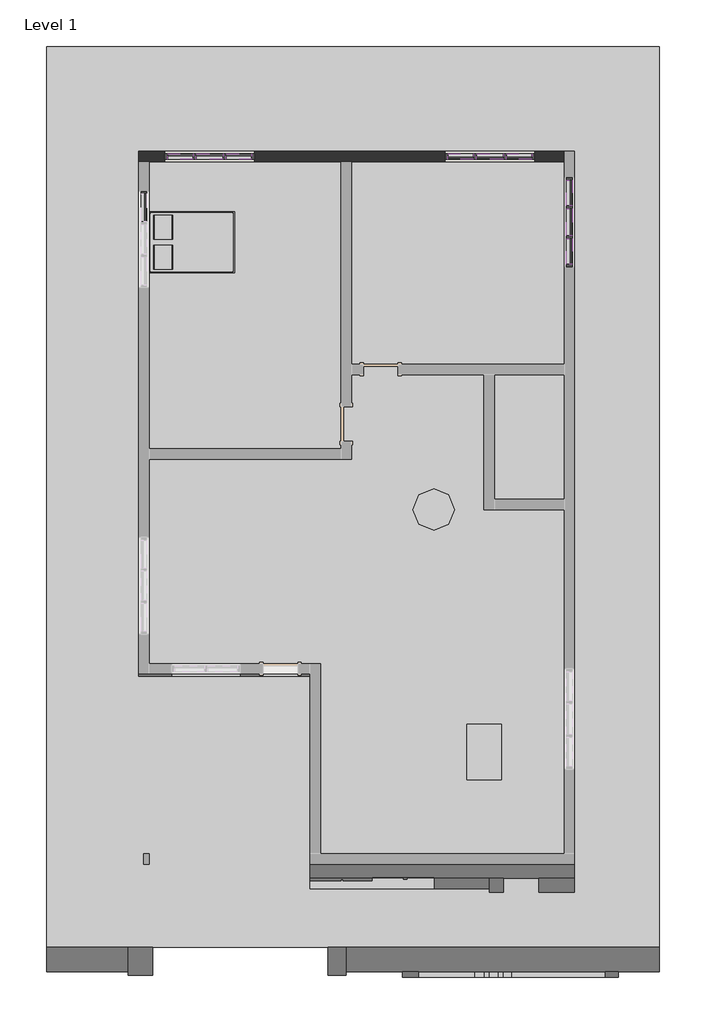
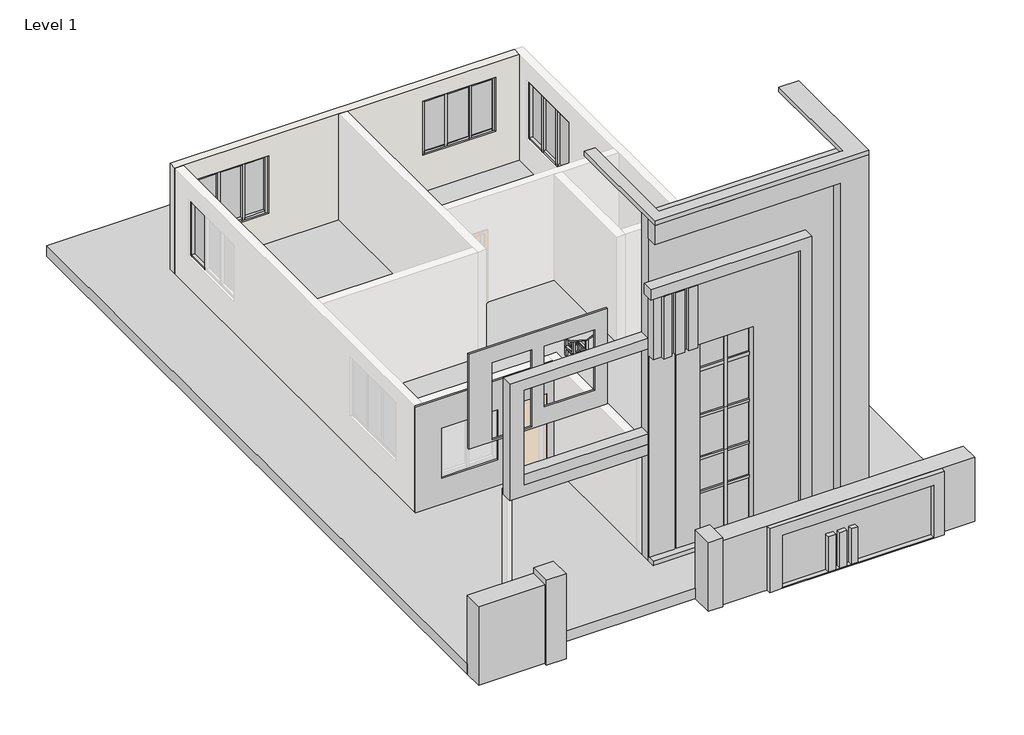
# One storey, part 2 of 2: 32 members, 10 plates, 3 furniture elements, 3 proxies, 1 wall.
"""IFC4 building model written with IfcOpenShell, lengths in millimetres."""

from ifc_helpers import new_model, si_unit, frame, origin, place, context, project, spatial, polyline, outline, extrude, faceted_brep, transform, mapped, element, save
from components import generic_models_1_generic_models_1_f513481b, generic_models_6_generic_models_6_42a028d1, furniture_b58f7881, furniture_acc2807d, furniture_52f35bf4, member_6f432376, member_a400357f, member_f14600c3, member_637ca32e, member_5ff6c43e, member_9389d775, member_1e31c4ff, member_d9b49a07, member_3f0e0172, member_8a463cd0, system_panel_glazed_0446ff67, system_panel_glazed_c50c6dba, system_panel_glazed_32442be8, system_panel_glazed_1c6e9dc7, system_panel_glazed_dfff3d37, system_panel_glazed_4691d008, system_panel_glazed_eebfb88d

model = new_model("IFC4")

# Units and contexts
model_context = context("Model", 3, world=origin())
ifc_project = project(units=[si_unit("LENGTHUNIT", "METRE", prefix="MILLI")], contexts=[model_context])

# Site, building, storey
site = spatial("IfcSite", under=ifc_project)
building = spatial("IfcBuilding", under=site)
storey = spatial("IfcBuildingStorey", under=building, Name="Level 1", Elevation=0.0)

# Proxies
placement = place(None, origin())
generic_models_1_generic_models_1_shape = generic_models_1_generic_models_1_f513481b(model_context)
element("IfcBuildingElementProxy", 1, Name="Generic Models 1 : Generic Models 1", ObjectType="Generic Models 1 : Generic Models 1", at=placement, inside=storey, context=model_context, shape_type="MappedRepresentation", body=[
    mapped(generic_models_1_generic_models_1_shape, transform((0.0, 0.0, 0.0), x_axis=(1.0, 0.0, 0.0), y_axis=(0.0, 1.0, 0.0), z_axis=(0.0, 0.0, 1.0))),
])
element("IfcBuildingElementProxy", 2, Name="Generic Models 2 : Generic Models 2", ObjectType="Generic Models 2 : Generic Models 2", at=placement, inside=storey, context=model_context, shape_type="SolidModel", body=[
    extrude(outline(polyline([(9822.6068762, -12103.529521), (9283.1169921, -12103.529521), (9283.1169921, -7061.629521), (0.0, -7061.629521), (0.0, -6274.229521), (9822.6068762, -6274.229521), (9822.6068762, -12103.529521)])), frame((0.0, -14950.4001929, 0.0), z_axis=(0.0, 1.0, 0.0), x_axis=(0.0, 0.0, 1.0)), (0.0, 0.0, 1.0), 304.8),
    extrude(outline(polyline([(8023.4485698, -12214.7903562), (7718.6485698, -12214.7903562), (7718.6485698, -8145.892021), (0.0, -8145.892021), (0.0, -7836.329521), (8023.4485698, -7836.329521), (8023.4485698, -12214.7903562)])), frame((0.0, -14950.4001929, 0.0), z_axis=(0.0, 1.0, 0.0), x_axis=(0.0, 0.0, 1.0)), (0.0, 0.0, 1.0), 304.8),
    faceted_brep([(-8153.829521, -14874.2001929, 7718.6485698), (-12103.529521, -14874.2001929, 7718.6485698), (-12103.529521, -14874.2001929, 5921.2879658), (-9360.329521, -14874.2001929, 5921.2879658), (-9360.329521, -14874.2001929, 130.0879658), (-12103.529521, -14874.2001929, 130.0879658), (-12103.529521, -14874.2001929, 0.0), (-8153.829521, -14874.2001929, 0.0), (-8153.829521, -14645.6001929, 7718.6485698), (-8153.829521, -14645.6001929, 0.0), (-12103.529521, -14645.6001929, 0.0), (-12103.529521, -14645.6001929, 7718.6485698), (-9360.329521, -14645.6001929, 130.0879658), (-9360.329521, -14645.6001929, 5921.2879658), (-10731.929521, -14645.6001929, 5921.2879658), (-10731.929521, -14645.6001929, 130.0879658), (-12103.529521, -14696.4001929, 130.0879658), (-12103.529521, -14696.4001929, 5921.2879658), (-11369.4072413, -14696.4001929, 5921.2879658), (-11369.4072413, -14696.4001929, 130.0879658), (-10731.929521, -14696.4001929, 130.0879658), (-10731.929521, -14696.4001929, 5921.2879658), (-11369.4072413, -14671.0001929, 130.0879658), (-11417.729521, -14671.0001929, 130.0879658), (-11417.729521, -14696.4001929, 130.0879658), (-11417.729521, -14696.4001929, 5921.2879658), (-11417.729521, -14671.0001929, 5921.2879658), (-11369.4072413, -14671.0001929, 5921.2879658)], [[[0, 1, 2, 3, 4, 5, 6, 7]], [[8, 9, 10, 11], [12, 13, 14, 15]], [[1, 0, 8, 11]], [[11, 10, 6, 5, 16, 17, 2, 1]], [[7, 6, 10, 9]], [[0, 7, 9, 8]], [[18, 19, 20, 21]], [[4, 3, 13, 12]], [[4, 12, 15, 20, 19, 22, 23, 24, 16, 5]], [[13, 3, 2, 17, 25, 26, 27, 18, 21, 14]], [[27, 26, 23, 22]], [[27, 22, 19, 18]], [[23, 26, 25, 24]], [[20, 15, 14, 21]], [[17, 16, 24, 25]]]),
    faceted_brep([(-6274.229521, -14645.6001929, 0.0), (-6274.229521, -14645.6001929, 9822.6068762), (-12103.529521, -14645.6001929, 9822.6068762), (-12103.529521, -14645.6001929, 0.0), (-9360.329521, -14645.6001929, 5921.2879658), (-9360.329521, -14645.6001929, 130.0879658), (-10731.929521, -14645.6001929, 130.0879658), (-10731.929521, -14645.6001929, 5921.2879658), (-6274.229521, -14340.8001929, 0.0), (-12103.529521, -14340.8001929, 0.0), (-12103.529521, -14340.8001929, 6400.8), (-12103.529521, -14340.8001929, 9822.6068762), (-6274.229521, -14340.8001929, 9822.6068762), (-6274.229521, -14340.8001929, 6400.8), (-9360.329521, -14620.2001929, 5921.2879658), (-10731.929521, -14620.2001929, 5921.2879658), (-10731.929521, -14620.2001929, 130.0879658), (-9360.329521, -14620.2001929, 130.0879658)], [[[0, 1, 2, 3], [4, 5, 6, 7]], [[8, 9, 10, 11, 12, 13]], [[1, 0, 8, 13, 12]], [[2, 1, 12, 11]], [[3, 2, 11, 10, 9]], [[0, 3, 9, 8]], [[14, 15, 16, 17]], [[14, 17, 5, 4]], [[17, 16, 6, 5]], [[16, 15, 7, 6]], [[15, 14, 4, 7]]]),
    extrude(outline(polyline([(-9969.4233324, -14671.0001929), (-10046.129521, -14671.0001929), (-10046.129521, -14620.2001929), (-9969.4233324, -14620.2001929), (-9969.4233324, -14671.0001929)])), frame((0.0, 0.0, 130.0879658), z_axis=(0.0, 0.0, 1.0), x_axis=(1.0, 0.0, 0.0)), (0.0, 0.0, 1.0), 5791.2),
    extrude(outline(polyline([(-9360.329521, -14671.0001929), (-10731.929521, -14671.0001929), (-10731.929521, -14620.2001929), (-9360.329521, -14620.2001929), (-9360.329521, -14671.0001929)])), frame((0.0, 0.0, 4975.7086338), z_axis=(0.0, 0.0, 1.0), x_axis=(1.0, 0.0, 0.0)), (0.0, 0.0, 1.0), 100.846843),
    extrude(outline(polyline([(-9360.329521, -14671.0001929), (-10731.929521, -14671.0001929), (-10731.929521, -14620.2001929), (-9360.329521, -14620.2001929), (-9360.329521, -14671.0001929)])), frame((0.0, 0.0, 3649.5165518), z_axis=(0.0, 0.0, 1.0), x_axis=(1.0, 0.0, 0.0)), (0.0, 0.0, 1.0), 71.0460044),
    extrude(outline(polyline([(-9360.329521, -14671.0001929), (-10731.929521, -14671.0001929), (-10731.929521, -14620.2001929), (-9360.329521, -14620.2001929), (-9360.329521, -14671.0001929)])), frame((0.0, 0.0, 2432.9915053), z_axis=(0.0, 0.0, 1.0), x_axis=(1.0, 0.0, 0.0)), (0.0, 0.0, 1.0), 63.6133902),
    extrude(outline(polyline([(-9360.329521, -14671.0001929), (-10731.929521, -14671.0001929), (-10731.929521, -14620.2001929), (-9360.329521, -14620.2001929), (-9360.329521, -14671.0001929)])), frame((0.0, 0.0, 1459.4738056), z_axis=(0.0, 0.0, 1.0), x_axis=(1.0, 0.0, 0.0)), (0.0, 0.0, 1.0), 65.6589833),
    extrude(outline(polyline([(-10945.1706491, -14975.8001929), (-11189.129521, -14975.8001929), (-11189.129521, -14874.2001929), (-10945.1706491, -14874.2001929), (-10945.1706491, -14975.8001929)])), frame((0.0, 0.0, 5921.2879658), z_axis=(0.0, 0.0, 1.0), x_axis=(1.0, 0.0, 0.0)), (0.0, 0.0, 1.0), 1797.360604),
    extrude(outline(polyline([(-11655.9903562, -14975.8001929), (-11874.929521, -14975.8001929), (-11874.929521, -14874.2001929), (-11655.9903562, -14874.2001929), (-11655.9903562, -14975.8001929)])), frame((0.0, 0.0, 5921.2879658), z_axis=(0.0, 0.0, 1.0), x_axis=(1.0, 0.0, 0.0)), (0.0, 0.0, 1.0), 1797.360604),
    extrude(outline(polyline([(-11297.3415593, -14975.8001929), (-11542.070497, -14975.8001929), (-11542.070497, -14874.2001929), (-11297.3415593, -14874.2001929), (-11297.3415593, -14975.8001929)])), frame((0.0, 0.0, 5921.2879658), z_axis=(0.0, 0.0, 1.0), x_axis=(1.0, 0.0, 0.0)), (0.0, 0.0, 1.0), 1797.360604),
    extrude(outline(polyline([(6096.0, -12103.529521), (6096.0, -15875.429521), (3352.8, -15875.429521), (3352.8, -12103.529521), (6096.0, -12103.529521)]), holes=[polyline([(3403.6, -15227.729521), (5613.4, -15227.729521), (5613.4, -14160.929521), (3403.6, -14160.929521), (3403.6, -15227.729521)]), polyline([(5594.0897089, -12446.429521), (3857.9365624, -12446.429521), (3857.9365624, -13818.029521), (5594.0897089, -13818.029521), (5594.0897089, -12446.429521)])]), frame((0.0, -12715.2001929, 0.0), z_axis=(0.0, 1.0, 0.0), x_axis=(0.0, 0.0, 1.0)), (0.0, 0.0, 1.0), 50.8),
    extrude(outline(polyline([(3048.0, -12103.529521), (3048.0, -15875.429521), (0.0, -15875.429521), (0.0, -12103.529521), (3048.0, -12103.529521)]), holes=[polyline([(2181.7525261, -13208.429521), (2181.7525261, -12294.029521), (50.8, -12294.029521), (50.8, -13208.429521), (2181.7525261, -13208.429521)]), polyline([(2181.7525261, -13627.529521), (750.5784943, -13627.529521), (750.5784943, -15151.529521), (2181.7525261, -15151.529521), (2181.7525261, -13627.529521)])]), frame((0.0, -10200.6001929, 0.0), z_axis=(0.0, 1.0, 0.0), x_axis=(0.0, 0.0, 1.0)), (0.0, 0.0, 1.0), 50.8),
    extrude(outline(polyline([(3352.8, -15487.5170157), (6096.0, -15487.5170157), (6096.0, -12103.529521), (6400.8, -12103.529521), (6400.8, -15875.429521), (3048.0, -15875.429521), (3048.0, -12103.529521), (3352.8, -12103.529521), (3352.8, -15487.5170157)])), frame((0.0, -14645.6001929, 0.0), z_axis=(0.0, 1.0, 0.0), x_axis=(0.0, 0.0, 1.0)), (0.0, 0.0, 1.0), 304.8),
    extrude(outline(polyline([(-12103.529521, -14340.8001929), (-12103.529521, -14645.6001929), (-15487.5170157, -14645.6001929), (-15487.5170157, -14340.8001929), (-12103.529521, -14340.8001929)])), frame((0.0, 0.0, 3352.8), z_axis=(0.0, 0.0, 1.0), x_axis=(1.0, 0.0, 0.0)), (0.0, 0.0, 1.0), 304.8),
])
generic_models_6_generic_models_6_shape = generic_models_6_generic_models_6_42a028d1(model_context)
element("IfcBuildingElementProxy", 3, Name="Generic Models 6 : Generic Models 6", ObjectType="Generic Models 6 : Generic Models 6", at=placement, inside=storey, context=model_context, shape_type="MappedRepresentation", body=[
    mapped(generic_models_6_generic_models_6_shape, transform((0.0, 0.0, 0.0), x_axis=(1.0, 0.0, 0.0), y_axis=(0.0, 1.0, 0.0), z_axis=(0.0, 0.0, 1.0))),
])

# Furniture
furniture_shape = furniture_b58f7881(model_context)
element("IfcFurniture", 4, ObjectType="Bed-Box : Double 53\" x 74\"", at=placement, inside=storey, context=model_context, shape_type="MappedRepresentation", body=[
    mapped(furniture_shape, transform((-14941.4590292, -989.3526519, 0.0), x_axis=(0.0, 1.0, 0.0), y_axis=(-1.0, 0.0, 0.0), z_axis=(0.0, 0.0, 1.0))),
])
furniture_2_shape = furniture_acc2807d(model_context)
element("IfcFurniture", 5, ObjectType="Table-Coffee Rectangular : 48\" x 30\"", at=placement, inside=storey, context=model_context, shape_type="MappedRepresentation", body=[
    mapped(furniture_2_shape, transform((-7898.5186892, -12477.6338232, 0.0), x_axis=(0.0, 1.0, 0.0), y_axis=(-1.0, 0.0, 0.0), z_axis=(0.0, 0.0, 1.0))),
])
furniture_3_shape = furniture_52f35bf4(model_context)
element("IfcFurniture", 6, ObjectType="Table-Dining Round w Chairs : 36\" Diameter", at=placement, inside=storey, context=model_context, shape_type="MappedRepresentation", body=[
    mapped(furniture_3_shape, transform((-9476.7114882, -6345.4215044, 0.0), x_axis=(1.0, 0.0, 0.0), y_axis=(0.0, 1.0, 0.0), z_axis=(0.0, 0.0, 1.0))),
])

# Members
member_shape = member_6f432376(model_context)
element("IfcMember", 7, ObjectType="Rectangular Mullion : 2.5\" x 5\" rectangular", at=placement, inside=storey, context=model_context, shape_type="MappedRepresentation", body=[
    mapped(member_shape, transform((-6388.529521, 156.2498071, 2498.2989313), x_axis=(0.0, 0.0, 1.0), y_axis=(-1.0, 0.0, 0.0), z_axis=(0.0, -1.0, 0.0))),
])
element("IfcMember", 8, ObjectType="Rectangular Mullion : 2.5\" x 5\" rectangular", at=placement, inside=storey, context=model_context, shape_type="MappedRepresentation", body=[
    mapped(member_shape, transform((-6388.529521, -1132.8001929, 2498.2989313), x_axis=(0.0, 0.0, 1.0), y_axis=(-1.0, 0.0, 0.0), z_axis=(0.0, -1.0, 0.0))),
])
element("IfcMember", 9, ObjectType="Rectangular Mullion : 2.5\" x 5\" rectangular", at=placement, inside=storey, context=model_context, shape_type="MappedRepresentation", body=[
    mapped(member_shape, transform((-7779.179521, 1242.0998071, 2608.4048272), x_axis=(0.0, 0.0, 1.0), y_axis=(0.0, 1.0, 0.0), z_axis=(-1.0, 0.0, 0.0))),
])
element("IfcMember", 10, ObjectType="Rectangular Mullion : 2.5\" x 5\" rectangular", at=placement, inside=storey, context=model_context, shape_type="MappedRepresentation", body=[
    mapped(member_shape, transform((-9068.229521, 1242.0998071, 2608.4048272), x_axis=(0.0, 0.0, 1.0), y_axis=(0.0, 1.0, 0.0), z_axis=(-1.0, 0.0, 0.0))),
])
element("IfcMember", 11, ObjectType="Rectangular Mullion : 2.5\" x 5\" rectangular", at=placement, inside=storey, context=model_context, shape_type="MappedRepresentation", body=[
    mapped(member_shape, transform((-14675.279521, 1242.0998071, 2518.5416429), x_axis=(0.0, 0.0, 1.0), y_axis=(0.0, -1.0, 0.0), z_axis=(1.0, 0.0, 0.0))),
])
element("IfcMember", 12, ObjectType="Rectangular Mullion : 2.5\" x 5\" rectangular", at=placement, inside=storey, context=model_context, shape_type="MappedRepresentation", body=[
    mapped(member_shape, transform((-13386.229521, 1242.0998071, 2518.5416429), x_axis=(0.0, 0.0, 1.0), y_axis=(0.0, -1.0, 0.0), z_axis=(1.0, 0.0, 0.0))),
])
member_2_shape = member_a400357f(model_context)
element("IfcMember", 13, ObjectType="Rectangular Mullion : 2.5\" x 5\" rectangular", at=placement, inside=storey, context=model_context, shape_type="MappedRepresentation", body=[
    mapped(member_2_shape, transform((-6388.529521, -504.1501929, 2498.2989313), x_axis=(0.0, 0.0, 1.0), y_axis=(-1.0, 0.0, 0.0), z_axis=(0.0, -1.0, 0.0))),
])
element("IfcMember", 14, ObjectType="Rectangular Mullion : 2.5\" x 5\" rectangular", at=placement, inside=storey, context=model_context, shape_type="MappedRepresentation", body=[
    mapped(member_2_shape, transform((-8439.579521, 1242.0998071, 2608.4048272), x_axis=(0.0, 0.0, 1.0), y_axis=(0.0, 1.0, 0.0), z_axis=(-1.0, 0.0, 0.0))),
])
element("IfcMember", 15, ObjectType="Rectangular Mullion : 2.5\" x 5\" rectangular", at=placement, inside=storey, context=model_context, shape_type="MappedRepresentation", body=[
    mapped(member_2_shape, transform((-14014.879521, 1242.0998071, 2518.5416429), x_axis=(0.0, 0.0, 1.0), y_axis=(0.0, -1.0, 0.0), z_axis=(1.0, 0.0, 0.0))),
])
member_3_shape = member_f14600c3(model_context)
element("IfcMember", 16, ObjectType="Rectangular Mullion : 2.5\" x 5\" rectangular", at=placement, inside=storey, context=model_context, shape_type="MappedRepresentation", body=[
    mapped(member_3_shape, transform((-6388.529521, 124.4998071, 812.0853055), x_axis=(0.0, -1.0, 0.0), y_axis=(-1.0, 0.0, 0.0), z_axis=(0.0, 0.0, -1.0))),
])
element("IfcMember", 17, ObjectType="Rectangular Mullion : 2.5\" x 5\" rectangular", at=placement, inside=storey, context=model_context, shape_type="MappedRepresentation", body=[
    mapped(member_3_shape, transform((-6388.529521, -535.9001929, 812.0853055), x_axis=(0.0, -1.0, 0.0), y_axis=(-1.0, 0.0, 0.0), z_axis=(0.0, 0.0, -1.0))),
])
element("IfcMember", 18, ObjectType="Rectangular Mullion : 2.5\" x 5\" rectangular", at=placement, inside=storey, context=model_context, shape_type="MappedRepresentation", body=[
    mapped(member_2_shape, transform((-6388.529521, 92.7498071, 812.0853055), x_axis=(0.0, 0.0, -1.0), y_axis=(-1.0, 0.0, 0.0), z_axis=(0.0, 1.0, 0.0))),
])
element("IfcMember", 19, ObjectType="Rectangular Mullion : 2.5\" x 5\" rectangular", at=placement, inside=storey, context=model_context, shape_type="MappedRepresentation", body=[
    mapped(member_2_shape, transform((-7842.679521, 1242.0998071, 1054.9476218), x_axis=(0.0, 0.0, -1.0), y_axis=(0.0, 1.0, 0.0), z_axis=(1.0, 0.0, 0.0))),
])
element("IfcMember", 20, ObjectType="Rectangular Mullion : 2.5\" x 5\" rectangular", at=placement, inside=storey, context=model_context, shape_type="MappedRepresentation", body=[
    mapped(member_2_shape, transform((-14611.779521, 1242.0998071, 854.6671361), x_axis=(0.0, 0.0, -1.0), y_axis=(0.0, -1.0, 0.0), z_axis=(-1.0, 0.0, 0.0))),
])
element("IfcMember", 21, ObjectType="Rectangular Mullion : 2.5\" x 5\" rectangular", at=placement, inside=storey, context=model_context, shape_type="MappedRepresentation", body=[
    mapped(member_shape, transform((-6388.529521, -567.6501929, 812.0853055), x_axis=(0.0, 0.0, -1.0), y_axis=(-1.0, 0.0, 0.0), z_axis=(0.0, 1.0, 0.0))),
])
element("IfcMember", 22, ObjectType="Rectangular Mullion : 2.5\" x 5\" rectangular", at=placement, inside=storey, context=model_context, shape_type="MappedRepresentation", body=[
    mapped(member_shape, transform((-6388.529521, 721.3998071, 812.0853055), x_axis=(0.0, 0.0, -1.0), y_axis=(-1.0, 0.0, 0.0), z_axis=(0.0, 1.0, 0.0))),
])
element("IfcMember", 23, ObjectType="Rectangular Mullion : 2.5\" x 5\" rectangular", at=placement, inside=storey, context=model_context, shape_type="MappedRepresentation", body=[
    mapped(member_shape, transform((-8503.079521, 1242.0998071, 1054.9476218), x_axis=(0.0, 0.0, -1.0), y_axis=(0.0, 1.0, 0.0), z_axis=(1.0, 0.0, 0.0))),
])
element("IfcMember", 24, ObjectType="Rectangular Mullion : 2.5\" x 5\" rectangular", at=placement, inside=storey, context=model_context, shape_type="MappedRepresentation", body=[
    mapped(member_shape, transform((-7214.029521, 1242.0998071, 1054.9476218), x_axis=(0.0, 0.0, -1.0), y_axis=(0.0, 1.0, 0.0), z_axis=(1.0, 0.0, 0.0))),
])
element("IfcMember", 25, ObjectType="Rectangular Mullion : 2.5\" x 5\" rectangular", at=placement, inside=storey, context=model_context, shape_type="MappedRepresentation", body=[
    mapped(member_shape, transform((-13951.379521, 1242.0998071, 854.6671361), x_axis=(0.0, 0.0, -1.0), y_axis=(0.0, -1.0, 0.0), z_axis=(-1.0, 0.0, 0.0))),
])
element("IfcMember", 26, ObjectType="Rectangular Mullion : 2.5\" x 5\" rectangular", at=placement, inside=storey, context=model_context, shape_type="MappedRepresentation", body=[
    mapped(member_shape, transform((-15240.429521, 1242.0998071, 854.6671361), x_axis=(0.0, 0.0, -1.0), y_axis=(0.0, -1.0, 0.0), z_axis=(-1.0, 0.0, 0.0))),
])
member_4_shape = member_637ca32e(model_context)
element("IfcMember", 27, ObjectType="Rectangular Mullion : 2.5\" x 5\" rectangular", at=placement, inside=storey, context=model_context, shape_type="MappedRepresentation", body=[
    mapped(member_4_shape, transform((-6388.529521, 784.8998071, 2498.2989313), x_axis=(0.0, 1.0, 0.0), y_axis=(-1.0, 0.0, 0.0), z_axis=(0.0, 0.0, 1.0))),
])
element("IfcMember", 28, ObjectType="Rectangular Mullion : 2.5\" x 5\" rectangular", at=placement, inside=storey, context=model_context, shape_type="MappedRepresentation", body=[
    mapped(member_4_shape, transform((-6388.529521, -1196.3001929, 812.0853055), x_axis=(0.0, -1.0, 0.0), y_axis=(-1.0, 0.0, 0.0), z_axis=(0.0, 0.0, -1.0))),
])
member_5_shape = member_5ff6c43e(model_context)
element("IfcMember", 29, ObjectType="Rectangular Mullion : 2.5\" x 5\" rectangular", at=placement, inside=storey, context=model_context, shape_type="MappedRepresentation", body=[
    mapped(member_5_shape, transform((-8471.329521, 1242.0998071, 1054.9476218), x_axis=(-1.0, 0.0, 0.0), y_axis=(0.0, 1.0, 0.0), z_axis=(0.0, 0.0, -1.0))),
])
element("IfcMember", 30, ObjectType="Rectangular Mullion : 2.5\" x 5\" rectangular", at=placement, inside=storey, context=model_context, shape_type="MappedRepresentation", body=[
    mapped(member_5_shape, transform((-7810.929521, 1242.0998071, 1054.9476218), x_axis=(-1.0, 0.0, 0.0), y_axis=(0.0, 1.0, 0.0), z_axis=(0.0, 0.0, -1.0))),
])
member_6_shape = member_9389d775(model_context)
element("IfcMember", 31, ObjectType="Rectangular Mullion : 2.5\" x 5\" rectangular", at=placement, inside=storey, context=model_context, shape_type="MappedRepresentation", body=[
    mapped(member_6_shape, transform((-9131.729521, 1242.0998071, 1054.9476218), x_axis=(-1.0, 0.0, 0.0), y_axis=(0.0, 1.0, 0.0), z_axis=(0.0, 0.0, -1.0))),
])
element("IfcMember", 32, ObjectType="Rectangular Mullion : 2.5\" x 5\" rectangular", at=placement, inside=storey, context=model_context, shape_type="MappedRepresentation", body=[
    mapped(member_6_shape, transform((-7150.529521, 1242.0998071, 2608.4048272), x_axis=(1.0, 0.0, 0.0), y_axis=(0.0, 1.0, 0.0), z_axis=(0.0, 0.0, 1.0))),
])
member_7_shape = member_1e31c4ff(model_context)
element("IfcMember", 33, ObjectType="Rectangular Mullion : 2.5\" x 5\" rectangular", at=placement, inside=storey, context=model_context, shape_type="MappedRepresentation", body=[
    mapped(member_7_shape, transform((-14643.529521, 1242.0998071, 854.6671361), x_axis=(1.0, 0.0, 0.0), y_axis=(0.0, -1.0, 0.0), z_axis=(0.0, 0.0, -1.0))),
])
element("IfcMember", 34, ObjectType="Rectangular Mullion : 2.5\" x 5\" rectangular", at=placement, inside=storey, context=model_context, shape_type="MappedRepresentation", body=[
    mapped(member_7_shape, transform((-13983.129521, 1242.0998071, 854.6671361), x_axis=(1.0, 0.0, 0.0), y_axis=(0.0, -1.0, 0.0), z_axis=(0.0, 0.0, -1.0))),
])
member_8_shape = member_d9b49a07(model_context)
element("IfcMember", 35, ObjectType="Rectangular Mullion : 2.5\" x 5\" rectangular", at=placement, inside=storey, context=model_context, shape_type="MappedRepresentation", body=[
    mapped(member_8_shape, transform((-15303.929521, 1242.0998071, 2518.5416429), x_axis=(-1.0, 0.0, 0.0), y_axis=(0.0, -1.0, 0.0), z_axis=(0.0, 0.0, 1.0))),
])
element("IfcMember", 36, ObjectType="Rectangular Mullion : 2.5\" x 5\" rectangular", at=placement, inside=storey, context=model_context, shape_type="MappedRepresentation", body=[
    mapped(member_8_shape, transform((-13322.729521, 1242.0998071, 854.6671361), x_axis=(1.0, 0.0, 0.0), y_axis=(0.0, -1.0, 0.0), z_axis=(0.0, 0.0, -1.0))),
])
member_9_shape = member_3f0e0172(model_context)
element("IfcMember", 37, ObjectType="Rectangular Mullion : 2.5\" x 5\" rectangular", at=placement, inside=storey, context=model_context, shape_type="MappedRepresentation", body=[
    mapped(member_9_shape, transform((-15761.129521, 416.5998071, 913.1300213), x_axis=(0.0, 0.0, -1.0), y_axis=(-1.0, 0.0, 0.0), z_axis=(0.0, 1.0, 0.0))),
])
member_10_shape = member_8a463cd0(model_context)
element("IfcMember", 38, ObjectType="Rectangular Mullion : 2.5\" x 5\" rectangular", at=placement, inside=storey, context=model_context, shape_type="MappedRepresentation", body=[
    mapped(member_10_shape, transform((-15761.129521, 480.0998071, 2533.943824), x_axis=(0.0, 1.0, 0.0), y_axis=(-1.0, 0.0, 0.0), z_axis=(0.0, 0.0, 1.0))),
])

# Plates
system_panel_glazed_shape = system_panel_glazed_0446ff67(model_context)
element("IfcPlate", 39, ObjectType="System Panel : Glazed", at=placement, inside=storey, context=model_context, shape_type="MappedRepresentation", body=[
    mapped(system_panel_glazed_shape, transform((-6388.529521, 438.8248071, 875.5853055), x_axis=(0.0, -1.0, 0.0), y_axis=(1.0, 0.0, 0.0), z_axis=(0.0, 0.0, 1.0))),
])
element("IfcPlate", 40, ObjectType="System Panel : Glazed", at=placement, inside=storey, context=model_context, shape_type="MappedRepresentation", body=[
    mapped(system_panel_glazed_shape, transform((-6388.529521, -850.2251929, 875.5853055), x_axis=(0.0, -1.0, 0.0), y_axis=(1.0, 0.0, 0.0), z_axis=(0.0, 0.0, 1.0))),
])
system_panel_glazed_2_shape = system_panel_glazed_c50c6dba(model_context)
element("IfcPlate", 41, ObjectType="System Panel : Glazed", at=placement, inside=storey, context=model_context, shape_type="MappedRepresentation", body=[
    mapped(system_panel_glazed_2_shape, transform((-6388.529521, -205.7001929, 875.5853055), x_axis=(0.0, -1.0, 0.0), y_axis=(1.0, 0.0, 0.0), z_axis=(0.0, 0.0, 1.0))),
])
system_panel_glazed_3_shape = system_panel_glazed_32442be8(model_context)
element("IfcPlate", 42, ObjectType="System Panel : Glazed", at=placement, inside=storey, context=model_context, shape_type="MappedRepresentation", body=[
    mapped(system_panel_glazed_3_shape, transform((-7496.604521, 1242.0998071, 1118.4476218), x_axis=(-1.0, 0.0, 0.0), y_axis=(0.0, -1.0, 0.0), z_axis=(0.0, 0.0, 1.0))),
])
element("IfcPlate", 43, ObjectType="System Panel : Glazed", at=placement, inside=storey, context=model_context, shape_type="MappedRepresentation", body=[
    mapped(system_panel_glazed_3_shape, transform((-8785.654521, 1242.0998071, 1118.4476218), x_axis=(-1.0, 0.0, 0.0), y_axis=(0.0, -1.0, 0.0), z_axis=(0.0, 0.0, 1.0))),
])
system_panel_glazed_4_shape = system_panel_glazed_1c6e9dc7(model_context)
element("IfcPlate", 44, ObjectType="System Panel : Glazed", at=placement, inside=storey, context=model_context, shape_type="MappedRepresentation", body=[
    mapped(system_panel_glazed_4_shape, transform((-8141.129521, 1242.0998071, 1118.4476218), x_axis=(-1.0, 0.0, 0.0), y_axis=(0.0, -1.0, 0.0), z_axis=(0.0, 0.0, 1.0))),
])
system_panel_glazed_5_shape = system_panel_glazed_dfff3d37(model_context)
element("IfcPlate", 45, ObjectType="System Panel : Glazed", at=placement, inside=storey, context=model_context, shape_type="MappedRepresentation", body=[
    mapped(system_panel_glazed_5_shape, transform((-14957.854521, 1242.0998071, 918.1671361), x_axis=(1.0, 0.0, 0.0), y_axis=(0.0, 1.0, 0.0), z_axis=(0.0, 0.0, 1.0))),
])
element("IfcPlate", 46, ObjectType="System Panel : Glazed", at=placement, inside=storey, context=model_context, shape_type="MappedRepresentation", body=[
    mapped(system_panel_glazed_5_shape, transform((-13668.804521, 1242.0998071, 918.1671361), x_axis=(1.0, 0.0, 0.0), y_axis=(0.0, 1.0, 0.0), z_axis=(0.0, 0.0, 1.0))),
])
system_panel_glazed_6_shape = system_panel_glazed_4691d008(model_context)
element("IfcPlate", 47, ObjectType="System Panel : Glazed", at=placement, inside=storey, context=model_context, shape_type="MappedRepresentation", body=[
    mapped(system_panel_glazed_6_shape, transform((-14313.329521, 1242.0998071, 918.1671361), x_axis=(1.0, 0.0, 0.0), y_axis=(0.0, 1.0, 0.0), z_axis=(0.0, 0.0, 1.0))),
])
system_panel_glazed_7_shape = system_panel_glazed_eebfb88d(model_context)
element("IfcPlate", 48, ObjectType="System Panel : Glazed", at=placement, inside=storey, context=model_context, shape_type="MappedRepresentation", body=[
    mapped(system_panel_glazed_7_shape, transform((-15761.129521, 108.6248071, 976.6300213), x_axis=(0.0, -1.0, 0.0), y_axis=(1.0, 0.0, 0.0), z_axis=(0.0, 0.0, 1.0))),
])

# Wall
element("IfcWall", 49, ObjectType="9\"", at=placement, inside=storey, context=model_context, shape_type="Brep", body=[
    faceted_brep([(-6502.829521, 1356.3998071, 0.0), (-15875.429521, 1356.3998071, 0.0), (-15875.429521, 1356.3998071, 3048.0), (-6502.829521, 1356.3998071, 3048.0), (-7150.529521, 1356.3998071, 1054.9476218), (-7150.529521, 1356.3998071, 2608.4048272), (-9131.729521, 1356.3998071, 2608.4048272), (-9131.729521, 1356.3998071, 1054.9476218), (-15303.929521, 1356.3998071, 2518.5416429), (-15303.929521, 1356.3998071, 854.6671361), (-13322.729521, 1356.3998071, 854.6671361), (-13322.729521, 1356.3998071, 2518.5416429), (-15875.429521, 1127.7998071, 0.0), (-15646.829521, 1127.7998071, 0.0), (-11417.729521, 1127.7998071, 0.0), (-11189.129521, 1127.7998071, 0.0), (-6502.829521, 1127.7998071, 0.0), (-6502.829521, 1127.7998071, 3048.0), (-11189.129521, 1127.7998071, 3048.0), (-11417.729521, 1127.7998071, 3048.0), (-15646.829521, 1127.7998071, 3048.0), (-15875.429521, 1127.7998071, 3048.0), (-7150.529521, 1127.7998071, 2608.4048272), (-7150.529521, 1127.7998071, 1054.9476218), (-9131.729521, 1127.7998071, 1054.9476218), (-9131.729521, 1127.7998071, 2608.4048272), (-15303.929521, 1127.7998071, 854.6671361), (-15303.929521, 1127.7998071, 2518.5416429), (-13322.729521, 1127.7998071, 2518.5416429), (-13322.729521, 1127.7998071, 854.6671361)], [[[0, 1, 2, 3], [4, 5, 6, 7], [8, 9, 10, 11]], [[12, 13, 14, 15, 16, 17, 18, 19, 20, 21], [22, 23, 24, 25], [26, 27, 28, 29]], [[1, 0, 16, 15, 14, 13, 12]], [[3, 2, 21, 20, 19, 18, 17]], [[0, 3, 17, 16]], [[2, 1, 12, 21]], [[4, 23, 22, 5]], [[5, 22, 25, 6]], [[6, 25, 24, 7]], [[23, 4, 7, 24]], [[26, 9, 8, 27]], [[27, 8, 11, 28]], [[10, 29, 28, 11]], [[9, 26, 29, 10]]]),
])

save(model, "model.ifc")

# Revit data of these elements
# Type "Bed-Box : Double 53\" x 74\""
#   Assembly Code = "E2020200"
#   Length = 6' - 2"
#   Width = 4' - 5"
#   Frame Material = Birch
#   Mattress Material = Linen, White
#   Default Elevation = 0
# Type "Table-Coffee Rectangular : 48\" x 30\""
#   Assembly Code = "E2020200"
#   Height = 1' - 1"
#   Length = 4' - 0"
#   Width = 2' - 6"
#   Base Material = Metal - Chrome
#   Table Top Material = Glass - Clear, Grey
#   Default Elevation = 0
# Type "Table-Dining Round w Chairs : 36\" Diameter"
#   Assembly Code = "E2020200"
#   Radius = 1' - 6"
#   Diameter = 3' - 0"
#   Height = 2' - 6"
#   Chairs = 4
#   Base Material = Pine
#   Top Material = Laminate, Linen, Matte
#   Default Elevation = 0
# Type "Rectangular Mullion : 2.5\" x 5\" rectangular"
#   built-in parameter 1007304 = 0.416667 (stored number, unit not read)
#   built-in parameter 1007301 = 0.104167 (stored number, unit not read)
#   built-in parameter 1007300 = 0.104167 (stored number, unit not read)
# Type "System Panel : Glazed"
#   Construction Type Id = "GSP4R"
#   Analytic Construction = "1/8 in Pilkington single glazing"
#   Visual Light Transmittance = 0.9
#   Solar Heat Gain Coefficient = 0.86
#   Heat Transfer Coefficient (U) = 1.18115 BTU/(h·ft²·°F)
#   Define Thermal Properties by = 1
# Type "9\""
#   Assembly Code = "B2010"
#   Layers, outside or top first: 0' - 9" no material (function 1)
# Element 1 (IfcBuildingElementProxy, "Generic Models 1 : Generic Models 1")
#   Phase Created = New Construction
# Element 2 (IfcBuildingElementProxy, "Generic Models 2 : Generic Models 2")
#   Phase Created = New Construction
# Element 3 (IfcBuildingElementProxy, "Generic Models 6 : Generic Models 6")
#   Phase Created = New Construction
# Element 4 (IfcFurniture, "Bed-Box : Double 53\" x 74\"")
#   Phase Created = New Construction
#   Materials on its faces: "Birch", "Linen, White"
# Element 5 (IfcFurniture, "Table-Coffee Rectangular : 48\" x 30\"")
#   Phase Created = New Construction
#   Materials on its faces: "Metal - Chrome", "Glass - Clear, Grey"
# Element 6 (IfcFurniture, "Table-Dining Round w Chairs : 36\" Diameter")
#   Phase Created = New Construction
#   Materials on its faces: "Pine", "Laminate, Linen, Matte"
# Elements 7, 8, 9, 10, 11, 12, 13, 14, 15, 16, 17, 18, 19, 20, 21, 22, 23, 24, 25, 26, 27, 28, 29, 30, 31, 32, 33, 34, 35, 36, 37, 38 (IfcMember, "Rectangular Mullion : 2.5\" x 5\" rectangular")
#   Phase Created = New Construction
#   Materials on its faces: "Aluminum"
# Elements 39, 40, 41, 42, 43, 44, 45, 46, 47, 48 (IfcPlate, "System Panel : Glazed")
#   Phase Created = New Construction
#   Materials on its faces: "Glass"
# Element 49 (IfcWall, "9\"")
#   Top Offset = 0' - 0"
#   Base Offset = 0' - 0"
#   Unconnected Height = 10' - 0"
#   wall height = 10' - 0"
#   Phase Created = New Construction
#   Base Constraint = Level 1
#   Materials on its faces: "Default Wall"
# Materials
#   "Birch": class "Wood", colour RGB 224 178 126, transparency 0, Description = "Betula Alleghaniensis", Cost = 0
#   "Linen, White": class "Textile", colour RGB 247 247 239, transparency 0, Description = "Linen, white", Cost = 0
#   "Metal - Chrome": colour RGB 57 57 57, transparency 0
#   "Glass - Clear, Grey": colour RGB 252 255 255, transparency 0.64
#   "Pine": class "Wood", colour RGB 223 192 134, transparency 0, Description = "Pinus Echinata", Cost = 0
#   "Laminate, Linen, Matte": class "Plastic", colour RGB 249 239 230, transparency 0, Description = "Plastic Laminate - Linen, Matte", Cost = 0
#   "Aluminum": class "Metal", colour RGB 247 247 247, transparency 0, Description = "Aluminum 6061", Cost = 0
#   "Glass": class "Glass", colour RGB 0 128 192, transparency 0.75, Description = "Soda Lime Glass", Cost = 0
#   "Default Wall": colour RGB 128 128 128, transparency 0, Cost = 0
